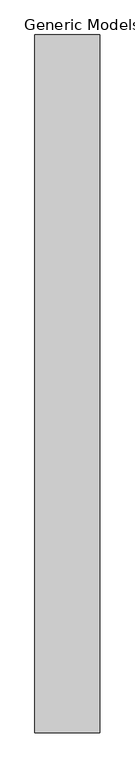
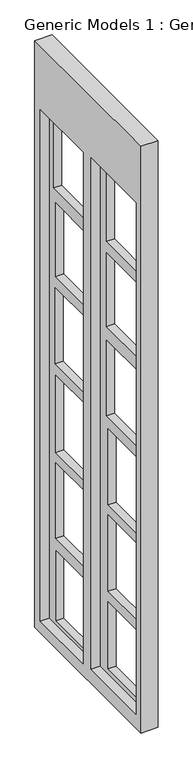
"""IFC4 building model written with IfcOpenShell, lengths in millimetres: proxy geometry, Generic Models 1 : Generic Models 1."""

from ifc_helpers import new_model, si_unit, origin, place, context, project, spatial, faceted_brep, source, transform, mapped, element, save


def generic_models_1_generic_models_1_14763b5c(model_context):
    return source(origin(), model_context, "Body", "Brep", [
        faceted_brep([(-6457.5487703, -3650.2683733, 20348.20716), (-6457.5487703, 2442.6962251, 20348.20716), (-7022.5256993, 2442.6962251, 20348.20716), (-7022.5256993, -3650.2683733, 20348.20716), (-6457.5487703, -3650.2683733, -158.4213758), (-7022.5256993, -3650.2683733, -158.4213758), (-7022.5256993, 2442.6962251, -158.4213758), (-6457.5487703, 2442.6962251, -158.4213758), (-6457.5487703, 80.4962251, 15427.4465317), (-6457.5487703, 80.4962251, 17896.0910797), (-6457.5487703, 1889.1429371, 17896.0910797), (-6457.5487703, 1889.1429371, 15427.4465317), (-6457.5487703, -8.6872134, 12397.0580072), (-6457.5487703, -8.6872134, 14967.2025866), (-6457.5487703, 1781.5076359, 14967.2025866), (-6457.5487703, 1781.5076359, 12397.0580072), (-6457.5487703, -17.3853235, 9328.6434489), (-6457.5487703, -17.3853235, 11990.9234937), (-6457.5487703, 1807.8390259, 11990.9234937), (-6457.5487703, 1807.8390259, 9328.6434489), (-6457.5487703, -30.6801441, 6248.4), (-6457.5487703, -30.6801441, 8955.1024994), (-6457.5487703, 1778.1125113, 8955.1024994), (-6457.5487703, 1778.1125113, 6248.4), (-6457.5487703, -22.1772395, 3249.0844472), (-6457.5487703, -22.1772395, 5902.7184846), (-6457.5487703, 1769.7396662, 5902.7184846), (-6457.5487703, 1769.7396662, 3249.0844472), (-6457.5487703, -35.8456262, 382.1575328), (-6457.5487703, -35.8456262, 2831.8492786), (-6457.5487703, 1759.3912226, 2831.8492786), (-6457.5487703, 1759.3912226, 382.1575328), (-6457.5487703, -3110.4760262, 15392.4), (-6457.5487703, -3110.4760262, 18001.2105755), (-6457.5487703, -1138.7037749, 18001.2105755), (-6457.5487703, -1138.7037749, 15392.4), (-6457.5487703, -3085.6925499, 12418.5246962), (-6457.5487703, -3085.6925499, 14992.0380524), (-6457.5487703, -1138.7037749, 14992.0380524), (-6457.5487703, -1138.7037749, 12418.5246962), (-6457.5487703, -3060.5044248, 9296.4), (-6457.5487703, -3060.5044248, 11945.6102001), (-6457.5487703, -1138.7037749, 11945.6102001), (-6457.5487703, -1138.7037749, 9296.4), (-6457.5487703, -3068.796499, 6248.4), (-6457.5487703, -3068.796499, 8900.8660013), (-6457.5487703, -1240.3037749, 8900.8660013), (-6457.5487703, -1240.3037749, 6248.4), (-6457.5487703, -3038.3259636, 3233.3282759), (-6457.5487703, -3038.3259636, 5897.9413451), (-6457.5487703, -1240.3037749, 5897.9413451), (-6457.5487703, -1240.3037749, 3233.3282759), (-6457.5487703, -3074.3445784, 518.8498071), (-6457.5487703, -3074.3445784, 2856.9721535), (-6457.5487703, -1240.3037749, 2856.9721535), (-6457.5487703, -1240.3037749, 518.8498071), (-7022.5256993, -312.6392341, 18107.7487565), (-7022.5256993, -312.6392341, 247.1582995), (-7022.5256993, 2136.1756814, 247.1582995), (-7022.5256993, 2136.1756814, 18107.7487565), (-7022.5256993, -3367.6830212, 18204.9064413), (-7022.5256993, -3367.6830212, 333.3375384), (-7022.5256993, -776.8830212, 333.3375384), (-7022.5256993, -776.8830212, 18204.9064413), (-6717.7256993, -312.6392341, 18107.7487565), (-6717.7256993, 2136.1756814, 18107.7487565), (-6717.7256993, 2136.1756814, 247.1582995), (-6717.7256993, -312.6392341, 247.1582995), (-6717.7256993, 80.4962251, 17896.0910797), (-6717.7256993, 80.4962251, 15427.4465317), (-6717.7256993, 1889.1429371, 15427.4465317), (-6717.7256993, 1889.1429371, 17896.0910797), (-6717.7256993, -8.6872134, 14967.2025866), (-6717.7256993, -8.6872134, 12397.0580072), (-6717.7256993, 1781.5076359, 12397.0580072), (-6717.7256993, 1781.5076359, 14967.2025866), (-6717.7256993, -17.3853235, 11990.9234937), (-6717.7256993, -17.3853235, 9328.6434489), (-6717.7256993, 1807.8390259, 9328.6434489), (-6717.7256993, 1807.8390259, 11990.9234937), (-6717.7256993, -30.6801441, 8955.1024994), (-6717.7256993, -30.6801441, 6248.4), (-6717.7256993, 1778.1125113, 6248.4), (-6717.7256993, 1778.1125113, 8955.1024994), (-6717.7256993, -22.1772395, 5902.7184846), (-6717.7256993, -22.1772395, 3249.0844472), (-6717.7256993, 1769.7396662, 3249.0844472), (-6717.7256993, 1769.7396662, 5902.7184846), (-6717.7256993, -35.8456262, 2831.8492786), (-6717.7256993, -35.8456262, 382.1575328), (-6717.7256993, 1759.3912226, 382.1575328), (-6717.7256993, 1759.3912226, 2831.8492786), (-6717.7256993, -3110.4760262, 15392.4), (-6717.7256993, -3110.4760262, 18001.2105755), (-6717.7256993, -1138.7037749, 15392.4), (-6717.7256993, -1138.7037749, 18001.2105755), (-6717.7256993, -3085.6925499, 12418.5246962), (-6717.7256993, -3085.6925499, 14992.0380524), (-6717.7256993, -1138.7037749, 12418.5246962), (-6717.7256993, -1138.7037749, 14992.0380524), (-6717.7256993, -3060.5044248, 9296.4), (-6717.7256993, -3060.5044248, 11945.6102001), (-6717.7256993, -1138.7037749, 9296.4), (-6717.7256993, -1138.7037749, 11945.6102001), (-6717.7256993, -3068.796499, 6248.4), (-6717.7256993, -3068.796499, 8900.8660013), (-6717.7256993, -1240.3037749, 6248.4), (-6717.7256993, -1240.3037749, 8900.8660013), (-6717.7256993, -3038.3259636, 3233.3282759), (-6717.7256993, -3038.3259636, 5897.9413451), (-6717.7256993, -1240.3037749, 3233.3282759), (-6717.7256993, -1240.3037749, 5897.9413451), (-6717.7256993, -3074.3445784, 518.8498071), (-6717.7256993, -3074.3445784, 2856.9721535), (-6717.7256993, -1240.3037749, 518.8498071), (-6717.7256993, -1240.3037749, 2856.9721535), (-6717.7256993, -3367.6830212, 18204.9064413), (-6717.7256993, -776.8830212, 18204.9064413), (-6717.7256993, -776.8830212, 333.3375384), (-6717.7256993, -3367.6830212, 333.3375384)], [[[0, 1, 2, 3]], [[4, 5, 6, 7]], [[1, 0, 4, 7], [8, 9, 10, 11], [12, 13, 14, 15], [16, 17, 18, 19], [20, 21, 22, 23], [24, 25, 26, 27], [28, 29, 30, 31], [32, 33, 34, 35], [36, 37, 38, 39], [40, 41, 42, 43], [44, 45, 46, 47], [48, 49, 50, 51], [52, 53, 54, 55]], [[2, 1, 7, 6]], [[3, 2, 6, 5], [56, 57, 58, 59], [60, 61, 62, 63]], [[0, 3, 5, 4]], [[64, 65, 66, 67], [68, 69, 70, 71], [72, 73, 74, 75], [76, 77, 78, 79], [80, 81, 82, 83], [84, 85, 86, 87], [88, 89, 90, 91]], [[64, 67, 57, 56]], [[67, 66, 58, 57]], [[66, 65, 59, 58]], [[65, 64, 56, 59]], [[68, 9, 8, 69]], [[69, 8, 11, 70]], [[70, 11, 10, 71]], [[9, 68, 71, 10]], [[72, 13, 12, 73]], [[73, 12, 15, 74]], [[74, 15, 14, 75]], [[13, 72, 75, 14]], [[76, 17, 16, 77]], [[77, 16, 19, 78]], [[78, 19, 18, 79]], [[17, 76, 79, 18]], [[80, 21, 20, 81]], [[81, 20, 23, 82]], [[82, 23, 22, 83]], [[21, 80, 83, 22]], [[84, 25, 24, 85]], [[85, 24, 27, 86]], [[86, 27, 26, 87]], [[25, 84, 87, 26]], [[88, 29, 28, 89]], [[89, 28, 31, 90]], [[90, 31, 30, 91]], [[29, 88, 91, 30]], [[33, 32, 92, 93]], [[32, 35, 94, 92]], [[35, 34, 95, 94]], [[34, 33, 93, 95]], [[37, 36, 96, 97]], [[36, 39, 98, 96]], [[39, 38, 99, 98]], [[38, 37, 97, 99]], [[41, 40, 100, 101]], [[40, 43, 102, 100]], [[43, 42, 103, 102]], [[42, 41, 101, 103]], [[45, 44, 104, 105]], [[44, 47, 106, 104]], [[47, 46, 107, 106]], [[46, 45, 105, 107]], [[49, 48, 108, 109]], [[48, 51, 110, 108]], [[51, 50, 111, 110]], [[50, 49, 109, 111]], [[53, 52, 112, 113]], [[52, 55, 114, 112]], [[55, 54, 115, 114]], [[54, 53, 113, 115]], [[116, 117, 118, 119], [93, 92, 94, 95], [97, 96, 98, 99], [101, 100, 102, 103], [105, 104, 106, 107], [109, 108, 110, 111], [113, 112, 114, 115]], [[116, 119, 61, 60]], [[119, 118, 62, 61]], [[118, 117, 63, 62]], [[117, 116, 60, 63]]]),
    ])


if __name__ == "__main__":
    model = new_model("IFC4")
    model_context = context("Model", 3, world=origin())
    ifc_project = project(units=[si_unit("LENGTHUNIT", "METRE", prefix="MILLI")], contexts=[model_context])
    site = spatial("IfcSite", under=ifc_project)
    building = spatial("IfcBuilding", under=site)
    placement = place(None, origin())
    generic_models_1_generic_models_1_shape = generic_models_1_generic_models_1_14763b5c(model_context)
    element("IfcBuildingElementProxy", 1, Name="Generic Models 1 : Generic Models 1", ObjectType="Generic Models 1 : Generic Models 1", at=placement, inside=building, context=model_context, shape_type="MappedRepresentation", body=[
        mapped(generic_models_1_generic_models_1_shape, transform((0.0, 0.0, 0.0), x_axis=(1.0, 0.0, 0.0), y_axis=(0.0, 1.0, 0.0), z_axis=(0.0, 0.0, 1.0))),
    ])
    save(model, "model.ifc")

# Revit data of these elements
# Element 1 (IfcBuildingElementProxy, "Generic Models 1 : Generic Models 1")
#   Materials on its faces: "Earth", "Door - Panel", "Door - Frame", "Grass"
# Materials
#   "Earth": class "Generic", colour RGB 97 75 62, transparency 0, Description = "Soil", Cost = 0
#   "Door - Panel": class "Wood", colour RGB 210 159 95, transparency 0, Cost = 0
#   "Door - Frame": colour RGB 118 70 51, transparency 0, Cost = 0
#   "Grass": class "Generic", colour RGB 104 137 66, transparency 0, Description = "Physical material.", Cost = 0
